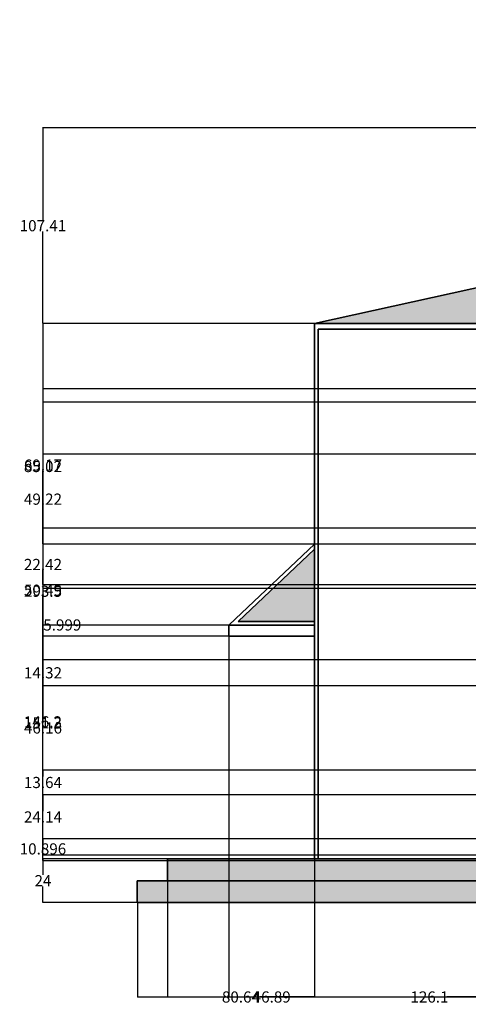
# Model space of a CAD drawing. Units: inches. Extents: x -655 to 499, y 20 to 616.
# Tile 1 of 7: x -655 to -409, y 20 to 560. Entities that reach past the tile are written whole.
import ezdxf

# ---------------------------------------------------------------- set-up
doc = ezdxf.new("R2010")
doc.units = ezdxf.units.IN
doc.header["$MEASUREMENT"] = 0
for name, color, linetype, lineweight in [('A-ANNO-DIMS', 2, 'Continuous', 18), ('A-ELEV', 7, 'Continuous', 35), ('A-ELEV-PATT', 9, 'Continuous', 13), ('A-ROOF', 1, 'Continuous', 35), ('C-TOPO', 18, 'Continuous', 18)]:
    doc.layers.add(name, color=color, linetype=linetype, lineweight=lineweight)
doc.styles.get("Standard").update_dxf_attribs({"font": 'arial.ttf'})
doc.dimstyles.get("Standard").update_dxf_attribs({"dimtxt": 6.125, "dimasz": 0.18, "dimexe": 0.18, "dimexo": 0.0625, "dimgap": 0.09, "dimtad": 0, "dimtih": 1, "dimtoh": 1, "dimdec": 4, "dimzin": 0, "dimdsep": 46, "dimlunit": 4, "dimtxsty": 'Standard', "dimcen": 0.09, "dimadec": 0, "dimazin": 0, "dimtfac": 1, "dimtdec": 4, "dimtofl": 0, "dimtmove": 0, "dimatfit": 3, "dimfxl": 1, "dimtolj": 1, "dimtzin": 0, "dimarcsym": 0})

# ---------------------------------------------------------------- blocks, each defined once
blk = doc.blocks.new('*D10')
at = {"layer": 'A-ANNO-DIMS', "color": 0, "lineweight": -2, "transparency": 16777216}
for p, q in [((434.11, 393.11), (434.11, 23.7)), ((-590.16, 75.57), (-590.16, 23.7)), ((-589.98, 23.88), (-90.54, 23.88)), ((433.93, 23.88), (-65.51, 23.88))]:
    blk.add_line(p, q, dxfattribs=at)
at = {"layer": 'A-ANNO-DIMS', "color": 0, "transparency": 16777216}
for points in [[(-589.98, 23.91), (-589.98, 23.85), (-590.16, 23.88)], [(433.93, 23.91), (433.93, 23.85), (434.11, 23.88)]]:
    blk.add_solid(points, dxfattribs=at)
at = {"layer": 'Defpoints', "color": 0, "transparency": 16777216}
for p in [(434.11, 393.17), (-590.16, 75.63), (434.11, 23.88)]:
    blk.add_point(p, dxfattribs=at)
at = {"layer": 'A-ANNO-DIMS', "color": 0, "transparency": 16777216, "insert": (-78.02, 23.88), "char_height": 6.125, "attachment_point": 5}
blk.add_mtext('\\A1;1024.3', dxfattribs=at)
blk = doc.blocks.new('*D11')
at = {"layer": 'A-ANNO-DIMS', "color": 0, "lineweight": -2, "transparency": 16777216}
for p, q in [((-573.68, 99.57), (-573.68, 23.7)), ((-493.03, 99.57), (-493.03, 23.7)), ((-573.5, 23.88), (-543.77, 23.88)), ((-493.21, 23.88), (-522.94, 23.88))]:
    blk.add_line(p, q, dxfattribs=at)
at = {"layer": 'A-ANNO-DIMS', "color": 0, "transparency": 16777216}
for points in [[(-573.5, 23.91), (-573.5, 23.85), (-573.68, 23.88)], [(-493.21, 23.91), (-493.21, 23.85), (-493.03, 23.88)]]:
    blk.add_solid(points, dxfattribs=at)
at = {"layer": 'Defpoints', "color": 0, "transparency": 16777216}
for p in [(-573.68, 99.63), (-493.03, 99.63), (-493.03, 23.88)]:
    blk.add_point(p, dxfattribs=at)
at = {"layer": 'A-ANNO-DIMS', "color": 0, "transparency": 16777216, "insert": (-533.36, 23.88), "char_height": 6.125, "attachment_point": 5}
blk.add_mtext('\\A1;80.64', dxfattribs=at)
blk = doc.blocks.new('*D12')
at = {"layer": 'A-ANNO-DIMS', "color": 0, "lineweight": -2, "transparency": 16777216}
for p, q in [((-493.03, 99.57), (-493.03, 23.7)), ((-366.94, 98.47), (-366.94, 23.7)), ((-492.85, 23.88), (-439.53, 23.88)), ((-367.12, 23.88), (-420.44, 23.88))]:
    blk.add_line(p, q, dxfattribs=at)
at = {"layer": 'A-ANNO-DIMS', "color": 0, "transparency": 16777216}
for points in [[(-492.85, 23.91), (-492.85, 23.85), (-493.03, 23.88)], [(-367.12, 23.91), (-367.12, 23.85), (-366.94, 23.88)]]:
    blk.add_solid(points, dxfattribs=at)
at = {"layer": 'Defpoints', "color": 0, "transparency": 16777216}
for p in [(-493.03, 99.63), (-366.94, 98.53), (-366.94, 23.88)]:
    blk.add_point(p, dxfattribs=at)
at = {"layer": 'A-ANNO-DIMS', "color": 0, "transparency": 16777216, "insert": (-429.99, 23.88), "char_height": 6.125, "attachment_point": 5}
blk.add_mtext('\\A1;126.1', dxfattribs=at)
blk = doc.blocks.new('*D21')
at = {"layer": 'A-ANNO-DIMS', "color": 0, "lineweight": -2, "transparency": 16777216}
for p, q in [((179.11, 559.78), (486.04, 559.78)), ((485.86, 559.6), (485.86, 320.92)), ((485.86, 75.81), (485.86, 314.49)), ((-590.1, 75.63), (486.04, 75.63))]:
    blk.add_line(p, q, dxfattribs=at)
at = {"layer": 'A-ANNO-DIMS', "color": 0, "transparency": 16777216}
for points in [[(485.83, 559.6), (485.89, 559.6), (485.86, 559.78)], [(485.83, 75.81), (485.89, 75.81), (485.86, 75.63)]]:
    blk.add_solid(points, dxfattribs=at)
at = {"layer": 'Defpoints', "color": 0, "transparency": 16777216}
for p in [(179.05, 559.78), (485.86, 559.78), (-590.16, 75.63)]:
    blk.add_point(p, dxfattribs=at)
at = {"layer": 'A-ANNO-DIMS', "color": 0, "transparency": 16777216, "insert": (485.86, 317.7), "char_height": 6.125, "attachment_point": 5}
blk.add_mtext('\\A1;484.15', dxfattribs=at)
blk = doc.blocks.new('*D22')
at = {"layer": 'A-ANNO-DIMS', "color": 0, "lineweight": -2, "transparency": 16777216}
for p, q in [((-5.81, 500.52), (-642.09, 500.52)), ((-641.91, 500.34), (-641.91, 450.03)), ((-641.91, 393.29), (-641.91, 443.6)), ((-493.1, 393.11), (-642.09, 393.11))]:
    blk.add_line(p, q, dxfattribs=at)
at = {"layer": 'A-ANNO-DIMS', "color": 0, "transparency": 16777216}
for points in [[(-641.94, 500.34), (-641.88, 500.34), (-641.91, 500.52)], [(-641.94, 393.29), (-641.88, 393.29), (-641.91, 393.11)]]:
    blk.add_solid(points, dxfattribs=at)
at = {"layer": 'Defpoints', "color": 0, "transparency": 16777216}
for p in [(-641.91, 500.52), (-5.74, 500.52), (-493.03, 393.11)]:
    blk.add_point(p, dxfattribs=at)
at = {"layer": 'A-ANNO-DIMS', "color": 0, "transparency": 16777216, "insert": (-641.91, 446.81), "char_height": 6.125, "attachment_point": 5}
blk.add_mtext('\\A1;107.41', dxfattribs=at)
blk = doc.blocks.new('*D23')
at = {"layer": 'A-ANNO-DIMS', "color": 0, "lineweight": -2, "transparency": 16777216}
for p, q in [((-493.1, 393.11), (-642.09, 393.11)), ((-641.91, 392.93), (-641.91, 249.59)), ((-641.91, 99.81), (-641.91, 243.15)), ((-573.74, 99.63), (-642.09, 99.63))]:
    blk.add_line(p, q, dxfattribs=at)
at = {"layer": 'A-ANNO-DIMS', "color": 0, "transparency": 16777216}
for points in [[(-641.94, 392.93), (-641.88, 392.93), (-641.91, 393.11)], [(-641.94, 99.81), (-641.88, 99.81), (-641.91, 99.63)]]:
    blk.add_solid(points, dxfattribs=at)
at = {"layer": 'Defpoints', "color": 0, "transparency": 16777216}
for p in [(-641.91, 393.11), (-493.03, 393.11), (-573.68, 99.63)]:
    blk.add_point(p, dxfattribs=at)
at = {"layer": 'A-ANNO-DIMS', "color": 0, "transparency": 16777216, "insert": (-641.91, 246.37), "char_height": 6.125, "attachment_point": 5}
blk.add_mtext('\\A1;293.5', dxfattribs=at)
blk = doc.blocks.new('*D24')
at = {"layer": 'A-ANNO-DIMS', "color": 0, "lineweight": -2, "transparency": 16777216}
for p, q in [((-573.74, 99.63), (-642.09, 99.63)), ((-641.91, 99.45), (-641.91, 90.79)), ((-641.91, 75.81), (-641.91, 84.46)), ((-590.23, 75.63), (-642.09, 75.63))]:
    blk.add_line(p, q, dxfattribs=at)
at = {"layer": 'A-ANNO-DIMS', "color": 0, "transparency": 16777216}
for points in [[(-641.94, 99.45), (-641.88, 99.45), (-641.91, 99.63)], [(-641.94, 75.81), (-641.88, 75.81), (-641.91, 75.63)]]:
    blk.add_solid(points, dxfattribs=at)
at = {"layer": 'Defpoints', "color": 0, "transparency": 16777216}
for p in [(-641.91, 99.63), (-573.68, 99.63), (-590.16, 75.63)]:
    blk.add_point(p, dxfattribs=at)
at = {"layer": 'A-ANNO-DIMS', "color": 0, "transparency": 16777216, "insert": (-641.91, 87.63), "char_height": 6.125, "attachment_point": 5}
blk.add_mtext('\\A1;24', dxfattribs=at)
blk = doc.blocks.new('*D25')
at = {"layer": 'A-ANNO-DIMS', "color": 0, "lineweight": -2, "transparency": 16777216}
for p, q in [((-399.44, 249.84), (-642.09, 249.84)), ((-641.91, 249.66), (-641.91, 177.41)), ((-641.91, 98.71), (-641.91, 170.97)), ((-367.01, 98.53), (-642.09, 98.53))]:
    blk.add_line(p, q, dxfattribs=at)
at = {"layer": 'A-ANNO-DIMS', "color": 0, "transparency": 16777216}
for points in [[(-641.94, 249.66), (-641.88, 249.66), (-641.91, 249.84)], [(-641.94, 98.71), (-641.88, 98.71), (-641.91, 98.53)]]:
    blk.add_solid(points, dxfattribs=at)
at = {"layer": 'Defpoints', "color": 0, "transparency": 16777216}
for p in [(-399.38, 249.84), (-641.91, 98.53), (-366.94, 98.53)]:
    blk.add_point(p, dxfattribs=at)
at = {"layer": 'A-ANNO-DIMS', "color": 0, "transparency": 16777216, "insert": (-641.91, 174.19), "char_height": 6.125, "attachment_point": 5}
blk.add_mtext('\\A1;151.3', dxfattribs=at)
blk = doc.blocks.new('*D26')
at = {"layer": 'A-ANNO-DIMS', "color": 0, "lineweight": -2, "transparency": 16777216}
for p, q in [((-355.49, 357.29), (-642.09, 357.29)), ((-641.91, 357.11), (-641.91, 317.99)), ((-641.91, 272.44), (-641.91, 311.56)), ((-355.49, 272.26), (-642.09, 272.26))]:
    blk.add_line(p, q, dxfattribs=at)
at = {"layer": 'A-ANNO-DIMS', "color": 0, "transparency": 16777216}
for points in [[(-641.94, 357.11), (-641.88, 357.11), (-641.91, 357.29)], [(-641.94, 272.44), (-641.88, 272.44), (-641.91, 272.26)]]:
    blk.add_solid(points, dxfattribs=at)
at = {"layer": 'Defpoints', "color": 0, "transparency": 16777216}
for p in [(-641.91, 357.29), (-355.43, 357.29), (-355.43, 272.26)]:
    blk.add_point(p, dxfattribs=at)
at = {"layer": 'A-ANNO-DIMS', "color": 0, "transparency": 16777216, "insert": (-641.91, 314.77), "char_height": 6.125, "attachment_point": 5}
blk.add_mtext('\\A1;85.02', dxfattribs=at)
blk = doc.blocks.new('*D34')
at = {"layer": 'A-ANNO-DIMS', "color": 0, "lineweight": -2, "transparency": 16777216}
for p, q in [((-347.1, 350.13), (-642.09, 350.13)), ((-641.91, 349.95), (-641.91, 318.77)), ((-641.91, 281.15), (-641.91, 312.33)), ((-347.1, 280.97), (-642.09, 280.97))]:
    blk.add_line(p, q, dxfattribs=at)
at = {"layer": 'A-ANNO-DIMS', "color": 0, "transparency": 16777216}
for points in [[(-641.94, 349.95), (-641.88, 349.95), (-641.91, 350.13)], [(-641.94, 281.15), (-641.88, 281.15), (-641.91, 280.97)]]:
    blk.add_solid(points, dxfattribs=at)
at = {"layer": 'Defpoints', "color": 0, "transparency": 16777216}
for p in [(-347.03, 350.13), (-641.91, 280.97), (-347.03, 280.97)]:
    blk.add_point(p, dxfattribs=at)
at = {"layer": 'A-ANNO-DIMS', "color": 0, "transparency": 16777216, "insert": (-641.91, 315.55), "char_height": 6.125, "attachment_point": 5}
blk.add_mtext('\\A1;69.17', dxfattribs=at)
blk = doc.blocks.new('*D36')
at = {"layer": 'A-ANNO-DIMS', "color": 0, "lineweight": -2, "transparency": 16777216}
for p, q in [((-399.44, 272.26), (-642.09, 272.26)), ((-641.91, 272.08), (-641.91, 264.22)), ((-641.91, 250.02), (-641.91, 257.89)), ((-399.44, 249.84), (-642.09, 249.84))]:
    blk.add_line(p, q, dxfattribs=at)
at = {"layer": 'A-ANNO-DIMS', "color": 0, "transparency": 16777216}
for points in [[(-641.94, 272.08), (-641.88, 272.08), (-641.91, 272.26)], [(-641.94, 250.02), (-641.88, 250.02), (-641.91, 249.84)]]:
    blk.add_solid(points, dxfattribs=at)
at = {"layer": 'Defpoints', "color": 0, "transparency": 16777216}
for p in [(-641.91, 272.26), (-399.38, 272.26), (-399.38, 249.84)]:
    blk.add_point(p, dxfattribs=at)
at = {"layer": 'A-ANNO-DIMS', "color": 0, "transparency": 16777216, "insert": (-641.91, 261.05), "char_height": 6.125, "attachment_point": 5}
blk.add_mtext('\\A1;22.42', dxfattribs=at)
blk = doc.blocks.new('*D37')
at = {"layer": 'A-ANNO-DIMS', "color": 0, "lineweight": -2, "transparency": 16777216}
for p, q in [((-402.14, 321.49), (-642.09, 321.49)), ((-641.91, 321.31), (-641.91, 300.09)), ((-641.91, 272.44), (-641.91, 293.66)), ((-399.44, 272.26), (-642.09, 272.26))]:
    blk.add_line(p, q, dxfattribs=at)
at = {"layer": 'A-ANNO-DIMS', "color": 0, "transparency": 16777216}
for points in [[(-641.94, 321.31), (-641.88, 321.31), (-641.91, 321.49)], [(-641.94, 272.44), (-641.88, 272.44), (-641.91, 272.26)]]:
    blk.add_solid(points, dxfattribs=at)
at = {"layer": 'Defpoints', "color": 0, "transparency": 16777216}
for p in [(-641.91, 321.49), (-402.07, 321.49), (-399.38, 272.26)]:
    blk.add_point(p, dxfattribs=at)
at = {"layer": 'A-ANNO-DIMS', "color": 0, "transparency": 16777216, "insert": (-641.91, 296.87), "char_height": 6.125, "attachment_point": 5}
blk.add_mtext('\\A1;49.22', dxfattribs=at)
blk = doc.blocks.new('*D50')
at = {"layer": 'A-ANNO-DIMS', "color": 0, "lineweight": -2, "transparency": 16777216}
for p, q in [((-354.42, 247.84), (-642.09, 247.84)), ((-641.91, 247.66), (-641.91, 177.95)), ((-641.91, 101.81), (-641.91, 171.52)), ((-354.42, 101.63), (-642.09, 101.63))]:
    blk.add_line(p, q, dxfattribs=at)
at = {"layer": 'A-ANNO-DIMS', "color": 0, "transparency": 16777216}
for points in [[(-641.94, 247.66), (-641.88, 247.66), (-641.91, 247.84)], [(-641.94, 101.81), (-641.88, 101.81), (-641.91, 101.63)]]:
    blk.add_solid(points, dxfattribs=at)
at = {"layer": 'Defpoints', "color": 0, "transparency": 16777216}
for p in [(-641.91, 247.84), (-354.35, 247.84), (-354.35, 101.63)]:
    blk.add_point(p, dxfattribs=at)
at = {"layer": 'A-ANNO-DIMS', "color": 0, "transparency": 16777216, "insert": (-641.91, 174.74), "char_height": 6.125, "attachment_point": 5}
blk.add_mtext('\\A1;146.2', dxfattribs=at)
blk = doc.blocks.new('*D52')
at = {"layer": 'A-ANNO-DIMS', "color": 0, "lineweight": -2, "transparency": 16777216}
for p, q in [((-539.92, 221.64), (-539.92, 23.7)), ((-493.03, 221.64), (-493.03, 23.7)), ((-539.74, 23.88), (-527.03, 23.88)), ((-493.21, 23.88), (-505.93, 23.88))]:
    blk.add_line(p, q, dxfattribs=at)
at = {"layer": 'A-ANNO-DIMS', "color": 0, "transparency": 16777216}
for points in [[(-539.74, 23.91), (-539.74, 23.85), (-539.92, 23.88)], [(-493.21, 23.91), (-493.21, 23.85), (-493.03, 23.88)]]:
    blk.add_solid(points, dxfattribs=at)
at = {"layer": 'Defpoints', "color": 0, "transparency": 16777216}
for p in [(-539.92, 221.7), (-493.03, 221.7), (-493.03, 23.88)]:
    blk.add_point(p, dxfattribs=at)
at = {"layer": 'A-ANNO-DIMS', "color": 0, "transparency": 16777216, "insert": (-516.48, 23.88), "char_height": 6.125, "attachment_point": 5}
blk.add_mtext('\\A1;46.89', dxfattribs=at)
blk = doc.blocks.new('*D53')
at = {"layer": 'A-ANNO-DIMS', "color": 0, "lineweight": -2, "transparency": 16777216}
for p, q in [((-493.1, 272.19), (-642.09, 272.19)), ((-641.91, 272.01), (-641.91, 250.16)), ((-641.91, 221.88), (-641.91, 243.73)), ((-539.99, 221.7), (-642.09, 221.7))]:
    blk.add_line(p, q, dxfattribs=at)
at = {"layer": 'A-ANNO-DIMS', "color": 0, "transparency": 16777216}
for points in [[(-641.94, 272.01), (-641.88, 272.01), (-641.91, 272.19)], [(-641.94, 221.88), (-641.88, 221.88), (-641.91, 221.7)]]:
    blk.add_solid(points, dxfattribs=at)
at = {"layer": 'Defpoints', "color": 0, "transparency": 16777216}
for p in [(-641.91, 272.19), (-493.03, 272.19), (-539.92, 221.7)]:
    blk.add_point(p, dxfattribs=at)
at = {"layer": 'A-ANNO-DIMS', "color": 0, "transparency": 16777216, "insert": (-641.91, 246.94), "char_height": 6.125, "attachment_point": 5}
blk.add_mtext('\\A1;50.49', dxfattribs=at)
blk = doc.blocks.new('*D54')
at = {"layer": 'A-ANNO-DIMS', "color": 0, "lineweight": -2, "transparency": 16777216}
for p, q in [((-539.99, 227.7), (-642.09, 227.7)), ((-641.91, 227.7), (-641.91, 227.88)), ((-641.91, 227.88), (-641.73, 227.88)), ((-641.91, 221.88), (-641.91, 227.52)), ((-539.99, 221.7), (-642.09, 221.7))]:
    blk.add_line(p, q, dxfattribs=at)
at = {"layer": 'A-ANNO-DIMS', "color": 0, "transparency": 16777216}
for points in [[(-641.94, 227.52), (-641.88, 227.52), (-641.91, 227.7)], [(-641.94, 221.88), (-641.88, 221.88), (-641.91, 221.7)]]:
    blk.add_solid(points, dxfattribs=at)
at = {"layer": 'Defpoints', "color": 0, "transparency": 16777216}
for p in [(-641.91, 227.7), (-539.92, 227.7), (-539.92, 221.7)]:
    blk.add_point(p, dxfattribs=at)
at = {"layer": 'A-ANNO-DIMS', "color": 0, "transparency": 16777216, "insert": (-631.3, 227.88), "char_height": 6.125, "attachment_point": 5}
blk.add_mtext('\\A1;5.999', dxfattribs=at)
blk = doc.blocks.new('*D67')
at = {"layer": 'A-ANNO-DIMS', "color": 0, "lineweight": -2, "transparency": 16777216}
for p, q in [((-42.36, 110.53), (-642.09, 110.53)), ((-641.91, 110.35), (-641.91, 108.29)), ((-64.18, 99.63), (-642.09, 99.63)), ((-641.91, 99.81), (-641.91, 101.86))]:
    blk.add_line(p, q, dxfattribs=at)
at = {"layer": 'A-ANNO-DIMS', "color": 0, "transparency": 16777216}
for points in [[(-641.94, 110.35), (-641.88, 110.35), (-641.91, 110.53)], [(-641.94, 99.81), (-641.88, 99.81), (-641.91, 99.63)]]:
    blk.add_solid(points, dxfattribs=at)
at = {"layer": 'Defpoints', "color": 0, "transparency": 16777216}
for p in [(-42.3, 110.53), (-641.91, 99.63), (-64.12, 99.63)]:
    blk.add_point(p, dxfattribs=at)
at = {"layer": 'A-ANNO-DIMS', "color": 0, "transparency": 16777216, "insert": (-641.91, 105.08), "char_height": 6.125, "attachment_point": 5}
blk.add_mtext('\\A1;10.896', dxfattribs=at)
blk = doc.blocks.new('*D68')
at = {"layer": 'A-ANNO-DIMS', "color": 0, "lineweight": -2, "transparency": 16777216}
for p, q in [((-42.36, 134.67), (-642.09, 134.67)), ((-641.91, 134.49), (-641.91, 125.76)), ((-641.91, 110.71), (-641.91, 119.43)), ((-42.36, 110.53), (-642.09, 110.53))]:
    blk.add_line(p, q, dxfattribs=at)
at = {"layer": 'A-ANNO-DIMS', "color": 0, "transparency": 16777216}
for points in [[(-641.94, 134.49), (-641.88, 134.49), (-641.91, 134.67)], [(-641.94, 110.71), (-641.88, 110.71), (-641.91, 110.53)]]:
    blk.add_solid(points, dxfattribs=at)
at = {"layer": 'Defpoints', "color": 0, "transparency": 16777216}
for p in [(-641.91, 134.67), (-42.3, 134.67), (-42.3, 110.53)]:
    blk.add_point(p, dxfattribs=at)
at = {"layer": 'A-ANNO-DIMS', "color": 0, "transparency": 16777216, "insert": (-641.91, 122.6), "char_height": 6.125, "attachment_point": 5}
blk.add_mtext('\\A1;24.14', dxfattribs=at)
blk = doc.blocks.new('*D69')
at = {"layer": 'A-ANNO-DIMS', "color": 0, "lineweight": -2, "transparency": 16777216}
for p, q in [((-42.36, 148.31), (-642.09, 148.31)), ((-641.91, 148.13), (-641.91, 144.71)), ((-641.91, 134.85), (-641.91, 138.27)), ((-42.36, 134.67), (-642.09, 134.67))]:
    blk.add_line(p, q, dxfattribs=at)
at = {"layer": 'A-ANNO-DIMS', "color": 0, "transparency": 16777216}
for points in [[(-641.94, 148.13), (-641.88, 148.13), (-641.91, 148.31)], [(-641.94, 134.85), (-641.88, 134.85), (-641.91, 134.67)]]:
    blk.add_solid(points, dxfattribs=at)
at = {"layer": 'Defpoints', "color": 0, "transparency": 16777216}
for p in [(-641.91, 148.31), (-42.3, 148.31), (-42.3, 134.67)]:
    blk.add_point(p, dxfattribs=at)
at = {"layer": 'A-ANNO-DIMS', "color": 0, "transparency": 16777216, "insert": (-641.91, 141.49), "char_height": 6.125, "attachment_point": 5}
blk.add_mtext('\\A1;13.64', dxfattribs=at)
blk = doc.blocks.new('*D70')
at = {"layer": 'A-ANNO-DIMS', "color": 0, "lineweight": -2, "transparency": 16777216}
for p, q in [((-42.36, 194.47), (-642.09, 194.47)), ((-641.91, 194.29), (-641.91, 174.61)), ((-641.91, 148.49), (-641.91, 168.17)), ((-42.36, 148.31), (-642.09, 148.31))]:
    blk.add_line(p, q, dxfattribs=at)
at = {"layer": 'A-ANNO-DIMS', "color": 0, "transparency": 16777216}
for points in [[(-641.94, 194.29), (-641.88, 194.29), (-641.91, 194.47)], [(-641.94, 148.49), (-641.88, 148.49), (-641.91, 148.31)]]:
    blk.add_solid(points, dxfattribs=at)
at = {"layer": 'Defpoints', "color": 0, "transparency": 16777216}
for p in [(-641.91, 194.47), (-42.3, 194.47), (-42.3, 148.31)]:
    blk.add_point(p, dxfattribs=at)
at = {"layer": 'A-ANNO-DIMS', "color": 0, "transparency": 16777216, "insert": (-641.91, 171.39), "char_height": 6.125, "attachment_point": 5}
blk.add_mtext('\\A1;46.16', dxfattribs=at)
blk = doc.blocks.new('*D71')
at = {"layer": 'A-ANNO-DIMS', "color": 0, "lineweight": -2, "transparency": 16777216}
for p, q in [((-64.18, 208.79), (-642.09, 208.79)), ((-641.91, 208.61), (-641.91, 204.85)), ((-42.36, 194.47), (-642.09, 194.47)), ((-641.91, 194.65), (-641.91, 198.41))]:
    blk.add_line(p, q, dxfattribs=at)
at = {"layer": 'A-ANNO-DIMS', "color": 0, "transparency": 16777216}
for points in [[(-641.94, 208.61), (-641.88, 208.61), (-641.91, 208.79)], [(-641.94, 194.65), (-641.88, 194.65), (-641.91, 194.47)]]:
    blk.add_solid(points, dxfattribs=at)
at = {"layer": 'Defpoints', "color": 0, "transparency": 16777216}
for p in [(-641.91, 208.79), (-64.12, 208.79), (-42.3, 194.47)]:
    blk.add_point(p, dxfattribs=at)
at = {"layer": 'A-ANNO-DIMS', "color": 0, "transparency": 16777216, "insert": (-641.91, 201.63), "char_height": 6.125, "attachment_point": 5}
blk.add_mtext('\\A1;14.32', dxfattribs=at)

msp = doc.modelspace()

# ---------------------------------------------------------------- hatches: boundary and pattern name
at = {"layer": 'A-ELEV-PATT'}
h = msp.add_hatch(color=256, dxfattribs=at)
h.dxf.hatch_style = 1
h.paths.add_polyline_path([(-126.8077, 93.6296), (-126.8077, 99.6296), (-145.6102, 99.6296), (-209.8047, 99.6296), (-366.9446, 98.5321), (-366.9446, 99.6296), (-506.835, 99.6296), (-573.6788, 99.6296), (-573.6788, 87.6296), (-506.835, 87.6296), (-161.7817, 87.6296), (-126.8077, 87.6296)])
h.paths.add_polyline_path([(419.8436, 99.6296), (99.4982, 99.6296), (99.4982, 87.6296), (419.8436, 87.6296)])
h.paths.add_polyline_path([(-100.4134, 99.6296), (-124.8077, 99.6296), (-124.8077, 93.6296), (-100.4134, 93.6296)])
h.paths.add_polyline_path([(-124.8077, 243.6296), (-126.8077, 243.6296), (-126.8077, 99.6296), (-124.8077, 99.6296)])
h.paths.add_polyline_path([(-124.8077, 99.6296), (-126.8077, 99.6296), (-126.8077, 93.6296), (-124.8077, 93.6296)])
at = {"layer": 'A-ROOF'}
h = msp.add_hatch(dxfattribs=at)
h.set_pattern_fill('AR-RSHKE', color=256)
h.paths.add_polyline_path([(-5.7434, 500.5192), (-493.0344, 393.1054), (-371.042, 393.1054), (119.6374, 393.1054), (415.7378, 393.1651)])
h.paths.add_polyline_path([(119.638, 282.9577), (-2.4978, 282.9577), (-133.531, 249.2017), (115.3098, 249.2518), (119.638, 250.1911)])
h.paths.add_polyline_path([(270.6361, 282.9577), (119.638, 282.9577), (119.638, 250.1911)], flags=17)
h.paths.add_polyline_path([(270.6361, 282.9577), (119.638, 250.1911), (119.638, 249.2527), (395.6741, 249.3083)])
h.paths.add_polyline_path([(-493.0344, 269.4313), (-534.9108, 229.7008), (-493.0344, 229.7008)])
at = {"layer": 'C-TOPO'}
h = msp.add_hatch(dxfattribs=at)
h.set_pattern_fill('GRAVEL', color=256, scale=2.2)
h.set_pattern_definition([(228.012788, (1.584, 2.2), (-17.6, -19.8), [0.295979, -29.301994]), (184.96974, (1.386, 1.98), (26.4, 2.2), [0.5079096, -50.2830345]), (132.510447, (0.88, 1.936), (22, -24.2), [0.3581336, -35.455272]), (267.27369, (0.022, 1.386), (2.2, 44), [0.4625236, -45.789828]), (292.833654, (0, 0.924), (-11, 26.4), [0.453541, -44.900621]), (357.27369, (0.176, 0.506), (-44, 2.2), [0.4625236, -45.789828]), (37.69424, (0.638, 0.484), (-28.6, -22), [0.611664, -60.554667]), (72.255328, (1.122, 0.858), (15.4, 48.4), [0.5774736, -57.169907]), (121.429566, (1.298, 1.408), (-17.6, 28.6), [0.46409, -45.944961]), (175.23636, (1.056, 1.804), (24.2, -2.2), [0.5298304, -25.961678]), (222.397438, (0.528, 1.848), (-26.4, -24.2), [0.6851856, -67.833425]), (138.814075, (2.2, 1.364), (-15.4, 13.2), [0.233862, -23.1524586]), (171.469234, (2.024, 1.518), (28.6, -4.4), [0.4449214, -44.047325]), (225, (1.584, 1.584), (-2e-16, -2.2), [0.311126, -2.800144]), (203.19859, (1.43, 1.848), (11, 4.4), [0.1675476, -16.587153]), (291.80141, (1.276, 1.782), (-2.2, 6.6), [0.2369466, -11.610416]), (30.96376, (1.364, 1.562), (6.6, 4.4), [0.384844, -12.44325]), (161.56505, (1.694, 1.76), (4.4, -2.2), [0.27828, -6.678731]), (16.38954, (0, 1.782), (22, 6.6), [0.38984, -38.594259]), (70.346176, (0.374, 1.892), (-8.8, -24.2), [0.327054, -32.378297]), (293.19859, (1.694, 2.2), (-4.4, 11), [0.335093, -16.419608]), (343.61046, (1.826, 1.892), (-22, 6.6), [0.38984, -38.594259]), (339.443955, (0, 0.418), (-11, 4.4), [0.375936, -18.420872]), (294.77514, (0.352, 0.286), (-11, 24.2), [0.3149916, -31.184215]), (66.80141, (1.716, 0), (4.4, 11), [0.335093, -16.419608]), (17.354025, (1.848, 0.308), (-28.6, -8.8), [0.368788, -36.509932]), (69.443955, (0.638, 0), (-4.4, -11), [0.187968, -18.60884]), (101.30993, (1.584, 0), (-2.2, 8.8), [0.112178, -11.105665]), (165.96376, (1.562, 0.11), (6.6, -2.2), [0.453541, -8.617291]), (186.009006, (1.122, 0.22), (22, 2.2), [0.42031, -41.610631]), (303.69007, (1.364, 1.364), (-2.2, 4.4), [0.3172884, -7.6149244]), (353.157227, (1.54, 1.1), (37.4, -4.4), [0.553947, -54.840638]), (60.945396, (2.09, 1.034), (-8.8, -15.4), [0.226503, -22.423883]), (90, (2.2, 1.232), (-2.2, 2.2), [0.132, -2.068]), (120.256437, (1.078, 0.286), (8.8, -15.4), [0.305633, -30.257744]), (48.012788, (0.924, 0.55), (17.6, 19.8), [0.5919584, -29.0060145]), (0, (1.32, 0.99), (2.2, 2.2), [0.572, -1.628]), (325.304846, (1.892, 0.99), (22, -15.4), [0.347851, -34.4372035]), (254.054604, (2.178, 0.792), (-2.2, -8.8), [0.3203244, -15.695917]), (207.645975, (2.09, 0.484), (-41.8, -22), [0.521543, -51.632843]), (175.426079, (1.628, 0.242), (-28.6, 2.2), [0.551758, -54.6239615])])
h.paths.add_polyline_path([(419.8436, 87.6296), (99.4982, 87.6296), (-161.7817, 87.6296), (-506.835, 87.6296), (-573.6788, 87.6296), (-590.1625, 87.6296), (-590.1625, 75.6296), (-496.5301, 75.6296), (-76.7836, 75.6296), (99.4982, 75.6296), (419.8436, 75.6296)])

# ---------------------------------------------------------------- linework, layer by layer
at = {"layer": 'A-ELEV'}
for p, q in [((-493.0344, 390.1054), (-493.0344, 99.6296)), ((-491.0344, 390.1054), (-491.0344, 99.6296)), ((-506.835, 99.6296), (-573.6788, 99.6296)), ((-573.6788, 99.6296), (-573.6788, 87.6296)), ((-145.6102, 99.6296), (-506.835, 99.6296)), ((-590.1625, 75.6296), (-590.1625, 87.6296)), ((-590.1625, 87.6296), (-573.6788, 87.6296)), ((-573.6788, 87.6296), (-506.835, 87.6296)), ((-161.7817, 87.6296), (-506.835, 87.6296)), ((-496.5301, 75.6296), (-590.1625, 75.6296)), ((-76.7836, 75.6296), (-496.5301, 75.6296))]:
    msp.add_line(p, q, dxfattribs=at)
at = {"layer": 'A-ROOF'}
for p, q in [((-493.0344, 393.1054), (-5.7434, 500.5192)), ((-493.0344, 390.1054), (-493.0344, 393.1054)), ((-322.5736, 390.1054), (-491.0344, 390.1054)), ((-493.0344, 272.1882), (-536.2874, 231.1517)), ((-493.0344, 269.4313), (-534.9108, 229.7008)), ((-536.2874, 231.1517), (-539.9247, 227.7008)), ((-539.9247, 227.7008), (-534.9108, 227.7008)), ((-539.9247, 227.7008), (-539.9247, 221.7016)), ((-534.9108, 229.7008), (-493.0344, 229.7008)), ((-534.9108, 227.7008), (-493.0344, 227.7008)), ((-539.9247, 221.7016), (-493.0344, 221.7016))]:
    msp.add_line(p, q, dxfattribs=at)
msp.add_lwpolyline([(432.6073, 393.1685), (119.6374, 393.1054), (-371.042, 393.1054), (-493.0344, 393.1054)], dxfattribs=at)

# ---------------------------------------------------------------- dimensions: what is measured, and where the dimension line sits
at = {"layer": 'A-ANNO-DIMS'}
for base, p1, p2, override, picture, middle in [((485.8637, 559.7795), (-590.1625, 75.6296), (179.0482, 559.7795), {"dimdec": 2, "dimlfac": 1, "dimrnd": 0, "dimzin": 0, "dimdsep": 46, "dimlunit": 2}, '*D21', (485.8637, 317.7046)), ((-641.9125, 500.5192), (-493.0344, 393.1054), (-5.7434, 500.5192), {"dimdec": 2, "dimlfac": 1, "dimrnd": 0, "dimzin": 0, "dimdsep": 46, "dimlunit": 2}, '*D22', (-641.9125, 446.8123)), ((-641.9125, 393.1054), (-573.6788, 99.6296), (-493.0344, 393.1054), {"dimdec": 1, "dimlfac": 1, "dimrnd": 0, "dimzin": 0, "dimdsep": 46, "dimlunit": 2}, '*D23', (-641.9125, 246.3675)), ((-641.9125, 357.2861), (-355.429, 272.2618), (-355.429, 357.2861), {"dimdec": 2, "dimlfac": 1, "dimrnd": 0, "dimzin": 0, "dimdsep": 46, "dimlunit": 2}, '*D26', (-641.9125, 314.7739)), ((-641.9125, 280.9678), (-347.0336, 350.1333), (-347.0336, 280.9678), {"dimdec": 2, "dimlfac": 1, "dimrnd": 0, "dimzin": 0, "dimdsep": 46, "dimlunit": 2}, '*D34', (-641.9125, 315.5506)), ((-641.9125, 321.4867), (-399.3758, 272.2618), (-402.0739, 321.4867), {"dimdec": 2, "dimlfac": 1, "dimrnd": 0, "dimzin": 0, "dimdsep": 46, "dimlunit": 2}, '*D37', (-641.9125, 296.8743)), ((-641.9125, 272.2618), (-399.3758, 249.8418), (-399.3758, 272.2618), {"dimdec": 2, "dimlfac": 1, "dimrnd": 0, "dimzin": 0, "dimdsep": 46, "dimlunit": 2}, '*D36', (-641.9125, 261.0518)), ((-641.9125, 272.1882), (-539.9247, 221.7016), (-493.0344, 272.1882), {"dimdec": 2, "dimlfac": 1, "dimrnd": 0, "dimzin": 0, "dimdsep": 46, "dimlunit": 2}, '*D53', (-641.9125, 246.9449)), ((-641.9125, 98.5321), (-399.3758, 249.8418), (-366.9446, 98.5321), {"dimdec": 1, "dimlfac": 1, "dimrnd": 0, "dimzin": 0, "dimdsep": 46, "dimlunit": 2}, '*D25', (-641.9125, 174.187)), ((-641.9125, 247.8418), (-354.3532, 101.6296), (-354.3532, 247.8418), {"dimdec": 1, "dimlfac": 1, "dimrnd": 0, "dimzin": 0, "dimdsep": 46, "dimlunit": 2}, '*D50', (-641.9125, 174.7357)), ((-641.9125, 227.7008), (-539.9247, 221.7016), (-539.9247, 227.7008), {"dimdec": 3, "dimlfac": 1, "dimrnd": 0, "dimzin": 0, "dimdsep": 46, "dimlunit": 2}, '*D54', (-631.3019, 227.8808)), ((-641.9125, 208.7923), (-42.2951, 194.4712), (-64.1158, 208.7923), {"dimdec": 2, "dimlfac": 1, "dimrnd": 0, "dimzin": 0, "dimdsep": 46, "dimlunit": 2}, '*D71', (-641.9125, 201.6317)), ((-641.9125, 194.4712), (-42.2951, 148.3082), (-42.2951, 194.4712), {"dimdec": 2, "dimlfac": 1, "dimrnd": 0, "dimzin": 0, "dimdsep": 46, "dimlunit": 2}, '*D70', (-641.9125, 171.3897)), ((-641.9125, 148.3082), (-42.2951, 134.6671), (-42.2951, 148.3082), {"dimdec": 2, "dimlfac": 1, "dimrnd": 0, "dimzin": 0, "dimdsep": 46, "dimlunit": 2}, '*D69', (-641.9125, 141.4877)), ((-641.9125, 134.6671), (-42.2951, 110.5254), (-42.2951, 134.6671), {"dimdec": 2, "dimlfac": 1, "dimrnd": 0, "dimzin": 0, "dimdsep": 46, "dimlunit": 2}, '*D68', (-641.9125, 122.5963)), ((-641.9125, 99.6296), (-42.2951, 110.5254), (-64.1158, 99.6296), {"dimdec": 3, "dimlfac": 1, "dimrnd": 0, "dimzin": 0, "dimdsep": 46, "dimlunit": 2}, '*D67', (-641.9125, 105.0775)), ((-641.9125, 99.6296), (-590.1625, 75.6296), (-573.6788, 99.6296), {"dimdec": 0, "dimlfac": 1, "dimrnd": 0, "dimzin": 0, "dimdsep": 46, "dimlunit": 2}, '*D24', (-641.9125, 87.6296))]:
    dim = msp.add_linear_dim(base=base, p1=p1, p2=p2, angle=90, dimstyle='Standard', override=override, dxfattribs=at)
    dim.commit()
    dim.dimension.update_dxf_attribs({"geometry": picture, "text_midpoint": middle})
for base, p1, p2, override, picture, middle in [((434.1137, 23.8796), (-590.1625, 75.6296), (434.1137, 393.1688), {"dimdec": 1, "dimlfac": 1, "dimrnd": 0, "dimzin": 0, "dimdsep": 46, "dimlunit": 2}, '*D10', (-78.0244, 23.8796)), ((-493.0344, 23.8796), (-539.9247, 221.7016), (-493.0344, 221.7016), {"dimdec": 2, "dimlfac": 1, "dimrnd": 0, "dimzin": 0, "dimdsep": 46, "dimlunit": 2}, '*D52', (-516.4795, 23.8796)), ((-493.0344, 23.8796), (-573.6788, 99.6296), (-493.0344, 99.6296), {"dimdec": 2, "dimlfac": 1, "dimrnd": 0, "dimzin": 0, "dimdsep": 46, "dimlunit": 2}, '*D11', (-533.3566, 23.8796)), ((-366.9446, 23.8796), (-493.0344, 99.6296), (-366.9446, 98.5321), {"dimdec": 1, "dimlfac": 1, "dimrnd": 0, "dimzin": 0, "dimdsep": 46, "dimlunit": 2}, '*D12', (-429.9895, 23.8796))]:
    dim = msp.add_linear_dim(base=base, p1=p1, p2=p2, dimstyle='Standard', override=override, dxfattribs=at)
    dim.commit()
    dim.dimension.update_dxf_attribs({"geometry": picture, "text_midpoint": middle})

doc.saveas('drawing.dxf')
